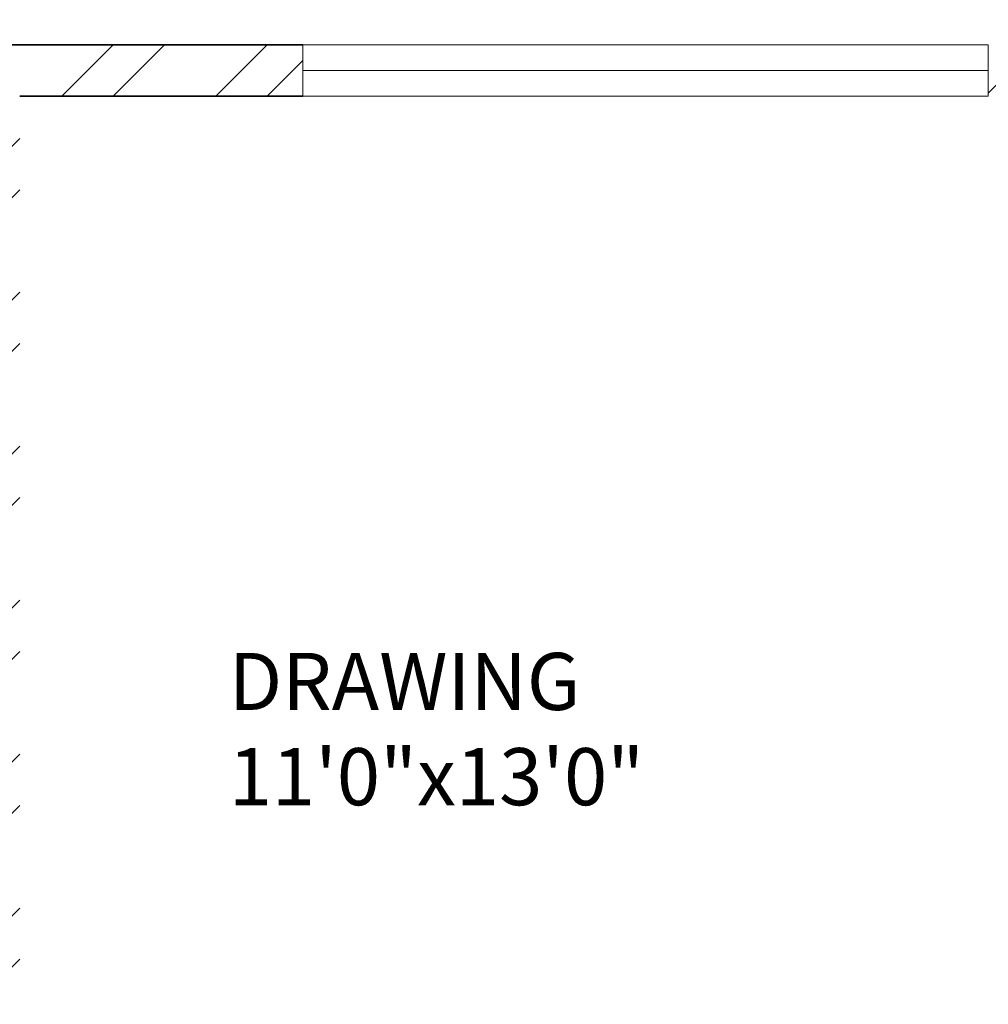
# Model space of a CAD drawing. Units: inches. Extents: x 1885 to 2748, y 783 to 2421.
# Tile 51 of 117: x 2311 to 2396, y 1764 to 1850. Entities that reach past the tile are written whole.
import ezdxf

# ---------------------------------------------------------------- set-up
doc = ezdxf.new("R2010")
doc.units = ezdxf.units.IN
for name, color, linetype, lineweight in [('A-AREA-IDEN', 7, 'Continuous', 18), ('A-GLAZ', 181, 'Continuous', 18), ('A-WALL', 7, 'Continuous', 35)]:
    doc.layers.add(name, color=color, linetype=linetype, lineweight=lineweight)
doc.layers.add('A-WALL-PATT', color=85, linetype='Continuous', lineweight=13, true_color=0x58ba48)
doc.styles.get("Standard").update_dxf_attribs({"font": 'arial.ttf'})

# ---------------------------------------------------------------- blocks, each defined once
blk = doc.blocks.new('WIN-60')
for p, q in [((0.004, 59.998), (4.504, 59.998)), ((0.004, 59.998), (0.004, -0.002)), ((4.504, 59.998), (2.254, 59.998)), ((2.254, 59.998), (2.254, -0.002)), ((4.504, -0.002), (4.504, 59.998)), ((2.254, -0.002), (0.004, -0.002)), ((0.004, -0.002), (4.504, -0.002))]:
    blk.add_line(p, q)

msp = doc.modelspace()

# ---------------------------------------------------------------- hatches: boundary and pattern name
at = {"layer": 'A-WALL-PATT'}
h = msp.add_hatch(dxfattribs=at)
h.set_pattern_fill('ANSI32', color=256)
h.paths.add_polyline_path([(2007.772, 2318.006), (1980.774, 2318.006), (1980.774, 2281.215), (1985.274, 2281.215), (1985.274, 2313.506), (2007.772, 2313.506), (2007.772, 2315.756)])
h.paths.add_polyline_path([(2094.324, 2318.006), (2067.772, 2318.006), (2067.772, 2313.506), (2094.324, 2313.506), (2094.324, 2315.756)])
h.paths.add_polyline_path([(2131.367, 2315.756), (2131.367, 2318.006), (2131.189, 2318.006), (2112.609, 2318.006), (2112.609, 2313.506), (2117.274, 2313.506), (2117.274, 2255.201), (2121.774, 2255.201), (2121.774, 2313.506), (2131.367, 2313.506)])
h.paths.add_polyline_path([(2190.512, 2318.006), (2155.367, 2318.006), (2155.367, 2313.506), (2169.774, 2313.506), (2169.774, 2229.506), (2121.774, 2229.506), (2121.774, 2233.451), (2119.524, 2233.451), (2117.274, 2233.451), (2117.274, 2201.101), (2121.774, 2201.101), (2121.774, 2225.006), (2169.774, 2225.006), (2169.774, 2165.006), (2306.274, 2165.006), (2306.274, 2066.006), (2310.774, 2066.006), (2344.274, 2066.006), (2486.274, 2066.006), (2486.274, 1886.006), (2483.02, 1886.006), (2483.02, 1881.506), (2486.274, 1881.506), (2486.274, 1880.678), (2490.774, 1880.678), (2490.774, 2070.506), (2344.274, 2070.506), (2310.774, 2070.506), (2310.774, 2165.006), (2310.774, 2173.636), (2308.524, 2173.636), (2306.274, 2173.636), (2306.274, 2169.506), (2174.274, 2169.506), (2174.274, 2313.506), (2190.512, 2313.506), (2190.512, 2315.756)])
h.paths.add_polyline_path([(1985.274, 2221.215), (1980.774, 2221.215), (1980.774, 2165.006), (1992.774, 2165.006), (1992.774, 2141.927), (1997.274, 2141.927), (1997.274, 2165.006), (2117.274, 2165.006), (2117.274, 2163.126), (2121.774, 2163.126), (2121.774, 2172.734), (2119.524, 2172.734), (2117.274, 2172.734), (2117.274, 2169.506), (1985.274, 2169.506)])
h.paths.add_polyline_path([(1997.274, 2105.927), (1992.774, 2105.927), (1992.774, 2070.506), (2016.774, 2070.506), (2016.774, 2059.123), (2019.024, 2059.123), (2021.274, 2059.123), (2021.274, 2070.506), (2117.274, 2070.506), (2117.274, 2022.506), (2114.423, 2022.506), (2114.423, 2018.006), (2123.627, 2018.006), (2123.627, 2020.256), (2123.627, 2022.506), (2121.774, 2022.506), (2121.774, 2142.587), (2119.524, 2142.587), (2117.274, 2142.587), (2117.274, 2075.006), (1997.274, 2075.006)])
h.paths.add_polyline_path([(2092.029, 2020.256), (2092.029, 2022.506), (2021.274, 2022.506), (2021.274, 2035.123), (2016.774, 2035.123), (2016.774, 2018.006), (2016.774, 1978.784), (2021.274, 1978.784), (2021.274, 2018.006), (2092.029, 2018.006)])
h.paths.add_polyline_path([(2260.938, 2022.506), (2153.105, 2022.506), (2153.105, 2020.256), (2153.105, 2018.006), (2155.274, 2018.006), (2155.274, 1886.006), (2107.629, 1886.006), (2107.629, 1881.506), (2182.911, 1881.506), (2182.911, 1883.756), (2182.911, 1886.006), (2159.774, 1886.006), (2159.774, 2018.006), (2260.938, 2018.006), (2260.938, 2020.256)])
h.paths.add_polyline_path([(2047.629, 1883.756), (2047.629, 1886.006), (2021.274, 1886.006), (2021.274, 1918.784), (2019.024, 1918.784), (2016.774, 1918.784), (2016.774, 1881.506), (2047.629, 1881.506)])
h.paths.add_polyline_path([(2306.361, 1883.756), (2306.361, 1886.006), (2296.274, 1886.006), (2296.274, 1982.006), (2316.535, 1982.006), (2316.535, 1984.256), (2316.535, 1986.506), (2296.274, 1986.506), (2296.274, 2022.506), (2289.276, 2022.506), (2289.276, 2018.006), (2291.774, 2018.006), (2291.774, 1886.006), (2242.911, 1886.006), (2242.911, 1881.506), (2306.361, 1881.506)], flags=17)
h.paths.add_polyline_path([(1985.274, 1843.006), (2021.6, 1843.006), (2021.534, 1845.441), (2021.477, 1847.506), (1980.774, 1847.506), (1980.774, 1809.446), (1985.274, 1809.446)])
h.paths.add_polyline_path([(2131.482, 1845.256), (2131.482, 1847.506), (2081.534, 1847.506), (2081.534, 1843.006), (2117.274, 1843.006), (2117.274, 1784.147), (2119.524, 1784.147), (2121.774, 1784.147), (2121.774, 1843.006), (2131.482, 1843.006)])
h.paths.add_polyline_path([(2203.886, 1847.506), (2155.482, 1847.506), (2155.482, 1843.006), (2169.774, 1843.006), (2169.774, 1759.006), (2121.774, 1759.006), (2121.774, 1761.457), (2117.274, 1761.457), (2117.274, 1730.429), (2121.774, 1730.429), (2121.774, 1754.506), (2177.421, 1754.506), (2177.421, 1756.756), (2177.421, 1759.006), (2174.274, 1759.006), (2174.274, 1843.006), (2203.886, 1843.006)])
h.paths.add_polyline_path([(2335.554, 1845.256), (2335.554, 1847.506), (2239.886, 1847.506), (2239.886, 1843.006), (2306.274, 1843.006), (2306.274, 1759.006), (2199.486, 1759.006), (2199.486, 1754.506), (2310.774, 1754.506), (2310.774, 1843.006), (2335.554, 1843.006)])
h.paths.add_polyline_path([(2348.774, 2022.506), (2344.274, 2022.506), (2344.274, 1986.506), (2341.681, 1986.506), (2341.681, 1982.006), (2344.274, 1982.006), (2344.274, 1886.006), (2330.361, 1886.006), (2330.361, 1881.506), (2361.627, 1881.506), (2361.627, 1883.756), (2361.627, 1886.006), (2348.774, 1886.006)], flags=17)
h.paths.add_polyline_path([(2283.251, 2315.756), (2283.251, 2318.006), (2238.512, 2318.006), (2238.512, 2313.506), (2283.251, 2313.506)], flags=17)
h.paths.add_polyline_path([(2363.274, 2348.006), (2388.677, 2348.006), (2388.677, 2350.256), (2388.677, 2352.506), (2358.774, 2352.506), (2358.774, 2348.006), (2358.774, 2318.006), (2344.481, 2318.006), (2344.481, 2313.506), (2358.774, 2313.506), (2358.774, 2229.506), (2310.774, 2229.506), (2310.774, 2231.952), (2306.274, 2231.952), (2306.274, 2205.611), (2310.774, 2205.611), (2310.774, 2225.006), (2358.774, 2225.006), (2358.774, 2211.506), (2452.329, 2211.506), (2452.329, 2213.756), (2452.329, 2216.006), (2363.274, 2216.006), (2363.274, 2318.006)])
h.paths.add_polyline_path([(2310.774, 2313.506), (2320.481, 2313.506), (2320.481, 2315.756), (2320.481, 2318.006), (2302.728, 2318.006), (2302.728, 2313.506), (2306.274, 2313.506), (2306.274, 2251.076), (2310.774, 2251.076)], flags=17)
h.paths.add_polyline_path([(2490.774, 2352.506), (2486.274, 2352.506), (2448.677, 2352.506), (2448.677, 2348.006), (2486.274, 2348.006), (2486.274, 2318.006), (2486.274, 2216.006), (2481.78, 2216.006), (2481.78, 2211.506), (2486.274, 2211.506), (2486.274, 2165.006), (2493.289, 2165.006), (2493.289, 2167.256), (2493.289, 2169.506), (2490.774, 2169.506), (2490.774, 2313.506), (2494.429, 2313.506), (2494.429, 2318.006), (2490.774, 2318.006)])
h.paths.add_polyline_path([(2534.653, 2318.006), (2515.691, 2318.006), (2515.691, 2313.506), (2534.653, 2313.506), (2534.653, 2315.756)])
h.paths.add_polyline_path([(2618.274, 2318.006), (2594.653, 2318.006), (2594.653, 2313.506), (2613.774, 2313.506), (2613.774, 2281.706), (2618.274, 2281.706)])
h.paths.add_polyline_path([(2618.274, 2221.706), (2613.774, 2221.706), (2613.774, 2169.506), (2554.019, 2169.506), (2554.019, 2165.006), (2613.774, 2165.006), (2613.774, 2152.878), (2618.274, 2152.878)])
h.paths.add_polyline_path([(2618.274, 2128.878), (2616.024, 2128.878), (2613.774, 2128.878), (2613.774, 2117.006), (2529.774, 2117.006), (2529.774, 2165.006), (2532.848, 2165.006), (2532.848, 2169.506), (2522.867, 2169.506), (2522.867, 2165.006), (2525.274, 2165.006), (2525.274, 2117.006), (2525.274, 2112.506), (2525.274, 2108.576), (2529.774, 2108.576), (2529.774, 2112.506), (2613.774, 2112.506), (2613.774, 2080.19), (2618.274, 2080.19)])
h.paths.add_polyline_path([(2618.274, 2044.19), (2616.024, 2044.19), (2613.774, 2044.19), (2613.774, 2015.506), (2529.774, 2015.506), (2529.774, 2088.582), (2527.524, 2088.582), (2525.274, 2088.582), (2525.274, 2011.006), (2613.774, 2011.006), (2613.774, 1956.755), (2618.274, 1956.755)])
h.paths.add_polyline_path([(2618.274, 1881.506), (2618.274, 1896.755), (2613.774, 1896.755), (2613.774, 1881.506), (2613.774, 1847.506), (2592.715, 1847.506), (2592.715, 1843.006), (2613.774, 1843.006), (2613.774, 1765.006), (2613.774, 1760.506), (2609.621, 1760.506), (2609.621, 1756.006), (2613.774, 1756.006), (2613.774, 1660.006), (2608.544, 1660.006), (2608.544, 1655.506), (2613.774, 1655.506), (2613.774, 1508.158), (2618.274, 1508.158)])
h.paths.add_polyline_path([(2565.774, 1843.006), (2568.997, 1843.006), (2568.997, 1847.506), (2490.774, 1847.506), (2490.774, 1849.7), (2488.524, 1849.7), (2486.274, 1849.7), (2486.274, 1847.506), (2477.274, 1847.506), (2477.274, 1838.506), (2477.274, 1821.493), (2486.274, 1821.493), (2486.274, 1838.506), (2561.274, 1838.506), (2561.274, 1765.006), (2486.274, 1765.006), (2486.274, 1786.157), (2477.274, 1786.157), (2477.274, 1765.006), (2477.274, 1756.006), (2486.274, 1756.006), (2565.774, 1756.006), (2585.621, 1756.006), (2585.621, 1758.256), (2585.621, 1760.506), (2565.774, 1760.506), (2565.774, 1765.006)])
h.paths.add_polyline_path([(2486.274, 1651.006), (2561.274, 1651.006), (2561.274, 1567.006), (2486.274, 1567.006), (2486.274, 1591.321), (2477.274, 1591.321), (2477.274, 1567.006), (2477.274, 1558.006), (2477.274, 1555.439), (2481.774, 1555.439), (2481.774, 1558.006), (2568.653, 1558.006), (2568.653, 1560.256), (2568.653, 1562.506), (2565.774, 1562.506), (2565.774, 1655.506), (2584.544, 1655.506), (2584.544, 1657.756), (2584.544, 1660.006), (2565.774, 1660.006), (2486.274, 1660.006), (2477.274, 1660.006), (2477.274, 1651.006), (2477.274, 1632.989), (2486.274, 1632.989)])
h.paths.add_polyline_path([(2449.967, 1883.756), (2449.967, 1886.006), (2421.627, 1886.006), (2421.627, 1881.506), (2449.967, 1881.506)], flags=17)
h.paths.add_polyline_path([(2447.274, 1847.506), (2395.554, 1847.506), (2395.554, 1843.006), (2442.774, 1843.006), (2442.774, 1809.27), (2447.274, 1809.27)])
h.paths.add_polyline_path([(1985.274, 1749.446), (1980.774, 1749.446), (1980.774, 1694.504), (1985.274, 1694.504), (1985.274, 1694.506), (1986.897, 1694.506), (1986.897, 1697.78), (1986.897, 1699.006), (1985.274, 1699.006)])
h.paths.add_polyline_path([(2152.774, 1699.006), (2121.774, 1699.006), (2121.774, 1703.668), (2119.524, 1703.668), (2117.274, 1703.668), (2117.274, 1699.006), (2009.219, 1699.006), (2009.219, 1694.506), (2148.274, 1694.506), (2148.274, 1692.631), (2152.774, 1692.631)])
h.paths.add_polyline_path([(2016.274, 1694.506), (2011.774, 1694.506), (2011.774, 1558.006), (2040.806, 1558.006), (2040.806, 1560.256), (2040.806, 1562.506), (2016.274, 1562.506)])
h.paths.add_polyline_path([(2152.774, 1663.017), (2150.524, 1663.017), (2148.274, 1663.017), (2148.274, 1562.506), (2100.806, 1562.506), (2100.806, 1558.006), (2165.119, 1558.006), (2165.119, 1560.256), (2165.119, 1562.506), (2152.774, 1562.506), (2152.774, 1610.506), (2224.774, 1610.506), (2224.774, 1607.99), (2229.274, 1607.99), (2229.274, 1615.006), (2152.774, 1615.006)])
h.paths.add_polyline_path([(2238.613, 1560.256), (2238.613, 1562.506), (2229.274, 1562.506), (2229.274, 1588.756), (2227.024, 1588.763), (2224.774, 1588.771), (2224.774, 1562.506), (2189.119, 1562.506), (2189.119, 1558.006), (2238.613, 1558.006)])
h.paths.add_polyline_path([(2336.024, 1560.256), (2336.024, 1562.506), (2310.774, 1562.506), (2310.774, 1656.347), (2308.524, 1656.347), (2306.274, 1656.347), (2306.274, 1562.506), (2286.613, 1562.506), (2286.613, 1558.006), (2336.024, 1558.006)])
h.paths.add_polyline_path([(2447.274, 1690.968), (2445.024, 1690.968), (2442.774, 1690.968), (2442.774, 1687.006), (2306.274, 1687.006), (2306.274, 1680.75), (2310.774, 1680.75), (2310.774, 1682.506), (2442.774, 1682.506), (2442.774, 1562.506), (2396.024, 1562.506), (2396.024, 1558.006), (2447.274, 1558.006)])
h.paths.add_polyline_path([(2447.274, 1749.27), (2445.024, 1749.27), (2442.774, 1749.27), (2442.774, 1717.232), (2447.274, 1717.232)])
h.paths.add_polyline_path([(2044.674, 1521.756), (2044.674, 1524.006), (2007.274, 1524.006), (2007.274, 1503.49), (2009.524, 1503.49), (2011.774, 1503.49), (2011.774, 1519.506), (2044.674, 1519.506)])
h.paths.add_polyline_path([(2177.969, 1521.756), (2177.969, 1524.006), (2104.674, 1524.006), (2104.674, 1519.506), (2145.774, 1519.506), (2145.774, 1387.506), (2143.37, 1387.506), (2143.37, 1383.006), (2251.585, 1383.006), (2251.585, 1385.256), (2251.585, 1387.506), (2150.274, 1387.506), (2150.274, 1519.506), (2177.969, 1519.506)])
h.paths.add_polyline_path([(2298.704, 1524.006), (2237.969, 1524.006), (2237.969, 1519.506), (2282.274, 1519.506), (2282.274, 1387.506), (2279.683, 1387.506), (2279.683, 1383.006), (2286.774, 1383.006), (2286.774, 1419.006), (2312.451, 1419.006), (2312.451, 1421.256), (2312.451, 1423.506), (2286.774, 1423.506), (2286.774, 1519.506), (2298.704, 1519.506), (2298.704, 1521.722)], flags=17)
h.paths.add_polyline_path([(2361.897, 1521.756), (2361.897, 1524.006), (2322.704, 1524.006), (2322.704, 1519.506), (2334.774, 1519.506), (2334.774, 1423.506), (2331.93, 1423.506), (2331.93, 1419.006), (2334.774, 1419.006), (2334.774, 1387.506), (2334.774, 1383.228), (2339.274, 1383.228), (2339.274, 1387.506), (2339.274, 1519.506), (2361.897, 1519.506)], flags=17)
h.paths.add_polyline_path([(2447.274, 1521.756), (2447.274, 1524.006), (2421.897, 1524.006), (2421.897, 1519.506), (2447.274, 1519.506)], flags=17)
h.paths.add_polyline_path([(2481.774, 1529.6), (2479.524, 1529.6), (2477.274, 1529.6), (2477.274, 1524.006), (2474.489, 1524.006), (2474.489, 1519.506), (2477.274, 1519.506), (2477.274, 1334.506), (2296.774, 1334.506), (2296.774, 1240.506), (2160.274, 1240.506), (2160.274, 1180.506), (2112.274, 1180.506), (2112.274, 1207.692), (2110.024, 1207.692), (2107.774, 1207.692), (2107.774, 1171.609), (2112.274, 1171.609), (2112.274, 1176.006), (2160.274, 1176.006), (2160.274, 1092.006), (2144.221, 1092.006), (2144.221, 1087.506), (2189.497, 1087.506), (2189.497, 1089.756), (2189.497, 1092.006), (2164.774, 1092.006), (2164.774, 1236.006), (2296.774, 1236.006), (2296.774, 1231.912), (2301.274, 1231.912), (2301.274, 1330.006), (2481.774, 1330.006), (2481.774, 1387.506)])
h.paths.add_polyline_path([(2618.274, 1448.158), (2613.774, 1448.158), (2613.774, 1382.506), (2529.774, 1382.506), (2525.274, 1382.506), (2525.274, 1307.062), (2529.774, 1307.062), (2529.774, 1378.006), (2613.774, 1378.006), (2613.774, 1354.988), (2618.274, 1354.988)])
h.paths.add_polyline_path([(2618.274, 1318.988), (2613.774, 1318.988), (2613.774, 1281.006), (2529.774, 1281.006), (2529.774, 1283.786), (2527.524, 1283.786), (2525.274, 1283.786), (2525.274, 1228.506), (2516.794, 1228.506), (2516.794, 1224.006), (2533.484, 1224.006), (2533.484, 1226.256), (2533.484, 1228.506), (2529.774, 1228.506), (2529.774, 1276.506), (2613.774, 1276.506), (2613.774, 1266.02), (2618.274, 1266.02)])
h.paths.add_polyline_path([(2618.274, 1134.964), (2613.774, 1134.964), (2613.774, 1092.006), (2594.545, 1092.006), (2594.545, 1087.506), (2618.274, 1087.506)])
h.paths.add_polyline_path([(2534.545, 1092.006), (2509.765, 1092.006), (2509.765, 1087.506), (2534.545, 1087.506), (2534.545, 1089.756)])
h.paths.add_polyline_path([(2481.274, 1224.006), (2484.117, 1224.006), (2484.117, 1226.256), (2484.117, 1228.506), (2476.774, 1228.506), (2476.774, 1198.506), (2471.61, 1198.506), (2471.61, 1194.006), (2476.774, 1194.006), (2476.774, 1062.006), (2436.894, 1062.006), (2436.894, 1057.506), (2476.774, 1057.506), (2481.274, 1057.506), (2481.274, 1062.006), (2481.274, 1087.506), (2485.354, 1087.506), (2485.354, 1089.756), (2485.354, 1092.006), (2481.274, 1092.006), (2481.274, 1117.506)])
h.paths.add_polyline_path([(2439.898, 1198.506), (2349.274, 1198.506), (2349.274, 1194.006), (2349.274, 1180.506), (2301.274, 1180.506), (2301.274, 1201.896), (2299.024, 1201.896), (2296.774, 1201.896), (2296.774, 1172.335), (2299.024, 1172.335), (2301.274, 1172.335), (2301.274, 1176.006), (2349.274, 1176.006), (2349.274, 1092.006), (2334.452, 1092.006), (2334.452, 1087.506), (2349.274, 1087.506), (2349.274, 1057.506), (2353.774, 1057.506), (2376.894, 1057.506), (2376.894, 1059.756), (2376.894, 1062.006), (2353.774, 1062.006), (2353.774, 1087.506), (2353.774, 1180.506), (2353.774, 1194.006), (2439.898, 1194.006), (2439.898, 1196.256)])
h.paths.add_polyline_path([(2270.596, 1089.756), (2270.596, 1092.006), (2249.497, 1092.006), (2249.497, 1087.506), (2270.596, 1087.506)], flags=17)
h.paths.add_polyline_path([(2310.452, 1092.006), (2301.274, 1092.006), (2301.274, 1153.292), (2296.774, 1153.292), (2296.774, 1092.006), (2293.786, 1092.006), (2293.786, 1087.506), (2310.452, 1087.506), (2310.452, 1089.756)], flags=17)
h.paths.add_polyline_path([(2112.274, 1150.328), (2110.024, 1150.328), (2107.774, 1150.328), (2107.774, 1092.006), (2104.465, 1092.006), (2104.465, 1087.506), (2120.221, 1087.506), (2120.221, 1089.756), (2120.221, 1092.006), (2112.274, 1092.006)])
h.paths.add_polyline_path([(2082.172, 1092.006), (2058.144, 1092.006), (2058.144, 1087.506), (2082.172, 1087.506), (2082.172, 1089.756)])
h.paths.add_polyline_path([(1975.774, 1145.638), (1971.274, 1145.638), (1971.274, 1087.506), (1980.774, 1087.506), (1998.144, 1087.506), (1998.144, 1089.756), (1998.144, 1092.006), (1985.274, 1092.006), (1975.774, 1092.006)])
h.paths.add_polyline_path([(2112.274, 1244.385), (2110.024, 1244.385), (2107.774, 1244.385), (2107.774, 1240.506), (1992.274, 1240.506), (1992.274, 1271.008), (1987.774, 1271.008), (1987.774, 1240.506), (1980.774, 1240.506), (1975.774, 1240.506), (1971.274, 1240.506), (1971.274, 1205.638), (1975.774, 1205.638), (1975.774, 1236.006), (2107.774, 1236.006), (2107.774, 1233.444), (2112.274, 1233.444), (2112.274, 1236.006)])
h.paths.add_polyline_path([(2112.274, 1383.006), (2114.783, 1383.006), (2114.783, 1385.256), (2114.783, 1387.506), (2102.476, 1387.506), (2102.476, 1383.006), (2107.774, 1383.006), (2107.774, 1335.006), (2011.774, 1335.006), (2011.774, 1349.939), (2007.274, 1349.939), (2007.274, 1335.006), (1987.774, 1335.006), (1987.774, 1330.506), (1987.774, 1307.008), (1992.274, 1307.008), (1992.274, 1330.506), (2007.274, 1330.506), (2107.774, 1330.506), (2107.774, 1264.711), (2112.274, 1264.711)])
h.paths.add_polyline_path([(2077.857, 1387.506), (2011.774, 1387.506), (2011.774, 1390.036), (2009.524, 1390.036), (2007.274, 1390.036), (2007.274, 1373.939), (2011.774, 1373.939), (2011.774, 1383.006), (2077.857, 1383.006)])
h.paths.add_polyline_path([(2011.774, 1443.49), (2007.274, 1443.49), (2007.274, 1410.248), (2011.774, 1410.248)])

# ---------------------------------------------------------------- linework, layer by layer
at = {"layer": 'A-WALL'}
for p, q in [((2239.886, 1847.506), (2335.554, 1847.506)), ((2310.774, 1843.006), (2335.554, 1843.006))]:
    msp.add_line(p, q, dxfattribs=at)

# ---------------------------------------------------------------- block references
at = {"layer": 'A-GLAZ', "extrusion": (0, 0, -1), "zscale": -1, "rotation": 90}
msp.add_blockref('WIN-60', (-2335.556, 1843.002), dxfattribs=at)

# ---------------------------------------------------------------- texts
at = {"layer": 'A-AREA-IDEN', "insert": (2329.064, 1794.287), "char_height": 5, "attachment_point": 1}
msp.add_mtext_dynamic_manual_height_columns('DRAWING\\P11\'0"x13\'0"', width=232.20962, gutter_width=12.5, heights=[0], dxfattribs=at)

doc.saveas('drawing.dxf')
